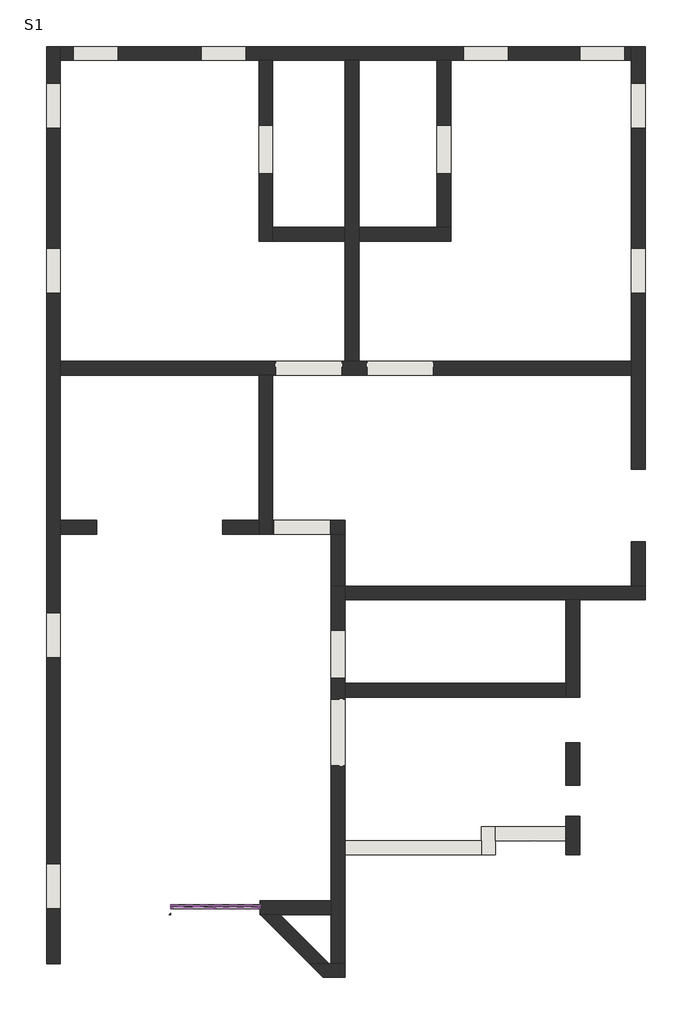
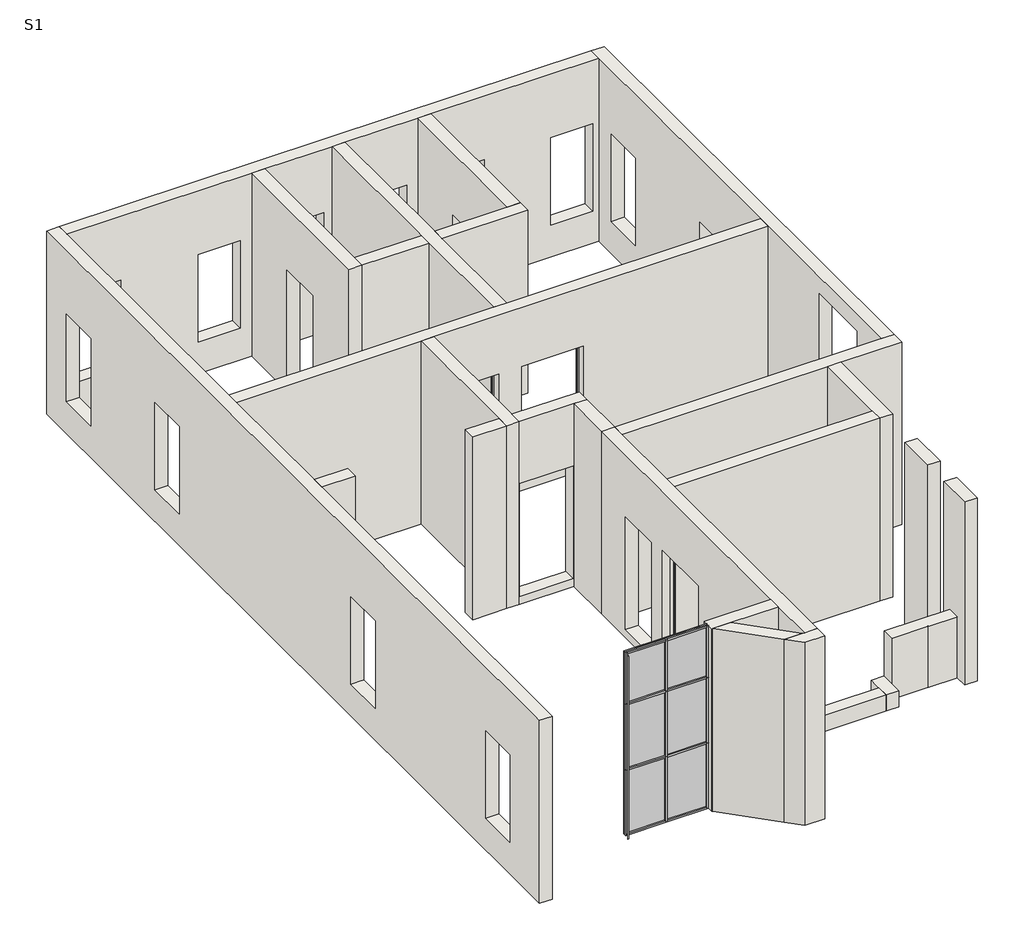
# One storey: 26 walls, 17 members, 6 plates.
"""IFC4 building model written with IfcOpenShell, lengths in millimetres."""

from ifc_helpers import new_model, si_unit, frame, origin, place, context, project, spatial, polyline, circle_curve, outline, extrude, faceted_brep, transform, mapped, element, save
from ifc_brep_helpers import plane_surface, revolved_surface, advanced_brep
from components import rectangular_mullion_30mm_square_a2edb205, rectangular_mullion_30mm_square_7d0e1db8, rectangular_mullion_30mm_square_4c7eb74d, rectangular_mullion_30mm_square_e6372653, rectangular_mullion_30mm_square_88df2287, rectangular_mullion_30mm_square_3df302c3, rectangular_mullion_30mm_square_038c5b05, rectangular_mullion_30mm_square_2b64bb93, system_panel_glazed_12388ada, system_panel_glazed_b614e8ed, system_panel_glazed_74337a84, system_panel_glazed_fe2b7919

model = new_model("IFC4")

# Units and contexts
model_context = context("Model", 3, world=origin())
ifc_project = project(units=[si_unit("LENGTHUNIT", "METRE", prefix="MILLI")], contexts=[model_context])

# Site, building, storey
site = spatial("IfcSite", under=ifc_project)
building = spatial("IfcBuilding", under=site)
storey = spatial("IfcBuildingStorey", under=building, Name="S1", Elevation=3750.0)

# Members
placement = place(None, origin())
rectangular_mullion_30mm_square_shape = rectangular_mullion_30mm_square_a2edb205(model_context)
element("IfcMember", 1, ObjectType="Rectangular Mullion : 30mm Square", at=placement, inside=storey, context=model_context, shape_type="MappedRepresentation", body=[
    mapped(rectangular_mullion_30mm_square_shape, transform((-6793.8712297, -9162.0014262, 7200.0), x_axis=(0.0, 0.0, 1.0), y_axis=(0.0, -1.0, 0.0), z_axis=(1.0, 0.0, 0.0))),
])
element("IfcMember", 2, ObjectType="Rectangular Mullion : 30mm Square", at=placement, inside=storey, context=model_context, shape_type="MappedRepresentation", body=[
    mapped(rectangular_mullion_30mm_square_shape, transform((-7498.8712297, -9162.0014262, 3750.0), x_axis=(0.0, 0.0, -1.0), y_axis=(0.0, -1.0, 0.0), z_axis=(-1.0, 0.0, 0.0))),
])
rectangular_mullion_30mm_square_2_shape = rectangular_mullion_30mm_square_7d0e1db8(model_context)
element("IfcMember", 3, ObjectType="Rectangular Mullion : 30mm Square", at=placement, inside=storey, context=model_context, shape_type="MappedRepresentation", body=[
    mapped(rectangular_mullion_30mm_square_2_shape, transform((-7513.8712297, -9162.0014262, 3750.0), x_axis=(1.0, 0.0, 0.0), y_axis=(0.0, -1.0, 0.0), z_axis=(0.0, 0.0, -1.0))),
])
rectangular_mullion_30mm_square_3_shape = rectangular_mullion_30mm_square_4c7eb74d(model_context)
element("IfcMember", 4, ObjectType="Rectangular Mullion : 30mm Square", at=placement, inside=storey, context=model_context, shape_type="MappedRepresentation", body=[
    mapped(rectangular_mullion_30mm_square_3_shape, transform((-6793.8712297, -9162.0014262, 6225.0), x_axis=(0.0, 0.0, 1.0), y_axis=(0.0, -1.0, 0.0), z_axis=(1.0, 0.0, 0.0))),
])
element("IfcMember", 5, ObjectType="Rectangular Mullion : 30mm Square", at=placement, inside=storey, context=model_context, shape_type="MappedRepresentation", body=[
    mapped(rectangular_mullion_30mm_square_3_shape, transform((-6793.8712297, -9162.0014262, 4987.5), x_axis=(0.0, 0.0, 1.0), y_axis=(0.0, -1.0, 0.0), z_axis=(1.0, 0.0, 0.0))),
])
element("IfcMember", 6, ObjectType="Rectangular Mullion : 30mm Square", at=placement, inside=storey, context=model_context, shape_type="MappedRepresentation", body=[
    mapped(rectangular_mullion_30mm_square_2_shape, transform((-7513.8712297, -9162.0014262, 4987.5), x_axis=(1.0, 0.0, 0.0), y_axis=(0.0, -1.0, 0.0), z_axis=(0.0, 0.0, -1.0))),
])
rectangular_mullion_30mm_square_4_shape = rectangular_mullion_30mm_square_e6372653(model_context)
element("IfcMember", 7, ObjectType="Rectangular Mullion : 30mm Square", at=placement, inside=storey, context=model_context, shape_type="MappedRepresentation", body=[
    mapped(rectangular_mullion_30mm_square_4_shape, transform((-6763.8712297, -9162.0014262, 3750.0), x_axis=(1.0, 0.0, 0.0), y_axis=(0.0, -1.0, 0.0), z_axis=(0.0, 0.0, -1.0))),
])
element("IfcMember", 8, ObjectType="Rectangular Mullion : 30mm Square", at=placement, inside=storey, context=model_context, shape_type="MappedRepresentation", body=[
    mapped(rectangular_mullion_30mm_square_4_shape, transform((-6763.8712297, -9162.0014262, 4987.5), x_axis=(1.0, 0.0, 0.0), y_axis=(0.0, -1.0, 0.0), z_axis=(0.0, 0.0, -1.0))),
])
element("IfcMember", 9, ObjectType="Rectangular Mullion : 30mm Square", at=placement, inside=storey, context=model_context, shape_type="MappedRepresentation", body=[
    mapped(rectangular_mullion_30mm_square_4_shape, transform((-8243.8712297, -9162.0014262, 6225.0), x_axis=(-1.0, 0.0, 0.0), y_axis=(0.0, -1.0, 0.0), z_axis=(0.0, 0.0, 1.0))),
])
element("IfcMember", 10, ObjectType="Rectangular Mullion : 30mm Square", at=placement, inside=storey, context=model_context, shape_type="MappedRepresentation", body=[
    mapped(rectangular_mullion_30mm_square_4_shape, transform((-8243.8712297, -9162.0014262, 4987.5), x_axis=(-1.0, 0.0, 0.0), y_axis=(0.0, -1.0, 0.0), z_axis=(0.0, 0.0, 1.0))),
])
rectangular_mullion_30mm_square_5_shape = rectangular_mullion_30mm_square_88df2287(model_context)
element("IfcMember", 11, ObjectType="Rectangular Mullion : 30mm Square", at=placement, inside=storey, context=model_context, shape_type="MappedRepresentation", body=[
    mapped(rectangular_mullion_30mm_square_5_shape, transform((-8213.8712297, -9162.0014262, 3750.0), x_axis=(0.0, 0.0, -1.0), y_axis=(0.0, -1.0, 0.0), z_axis=(-1.0, 0.0, 0.0))),
])
rectangular_mullion_30mm_square_6_shape = rectangular_mullion_30mm_square_3df302c3(model_context)
element("IfcMember", 12, ObjectType="Rectangular Mullion : 30mm Square", at=placement, inside=storey, context=model_context, shape_type="MappedRepresentation", body=[
    mapped(rectangular_mullion_30mm_square_6_shape, transform((-7528.8712297, -9162.0014262, 6225.0), x_axis=(0.0, 0.0, 1.0), y_axis=(0.0, -1.0, 0.0), z_axis=(1.0, 0.0, 0.0))),
])
element("IfcMember", 13, ObjectType="Rectangular Mullion : 30mm Square", at=placement, inside=storey, context=model_context, shape_type="MappedRepresentation", body=[
    mapped(rectangular_mullion_30mm_square_6_shape, transform((-7528.8712297, -9162.0014262, 4987.5), x_axis=(0.0, 0.0, 1.0), y_axis=(0.0, -1.0, 0.0), z_axis=(1.0, 0.0, 0.0))),
])
element("IfcMember", 14, ObjectType="Rectangular Mullion : 30mm Square", at=placement, inside=storey, context=model_context, shape_type="MappedRepresentation", body=[
    mapped(rectangular_mullion_30mm_square_5_shape, transform((-7528.8712297, -9162.0014262, 7200.0), x_axis=(0.0, 0.0, 1.0), y_axis=(0.0, -1.0, 0.0), z_axis=(1.0, 0.0, 0.0))),
])
rectangular_mullion_30mm_square_7_shape = rectangular_mullion_30mm_square_038c5b05(model_context)
element("IfcMember", 15, ObjectType="Rectangular Mullion : 30mm Square", at=placement, inside=storey, context=model_context, shape_type="MappedRepresentation", body=[
    mapped(rectangular_mullion_30mm_square_7_shape, transform((-7513.8712297, -9162.0014262, 6225.0), x_axis=(1.0, 0.0, 0.0), y_axis=(0.0, -1.0, 0.0), z_axis=(0.0, 0.0, -1.0))),
])
rectangular_mullion_30mm_square_8_shape = rectangular_mullion_30mm_square_2b64bb93(model_context)
element("IfcMember", 16, ObjectType="Rectangular Mullion : 30mm Square", at=placement, inside=storey, context=model_context, shape_type="MappedRepresentation", body=[
    mapped(rectangular_mullion_30mm_square_8_shape, transform((-8243.8712297, -9162.0014262, 7200.0), x_axis=(-1.0, 0.0, 0.0), y_axis=(0.0, -1.0, 0.0), z_axis=(0.0, 0.0, 1.0))),
])
element("IfcMember", 17, ObjectType="Rectangular Mullion : 30mm Square", at=placement, inside=storey, context=model_context, shape_type="MappedRepresentation", body=[
    mapped(rectangular_mullion_30mm_square_8_shape, transform((-6763.8712297, -9162.0014262, 6225.0), x_axis=(1.0, 0.0, 0.0), y_axis=(0.0, -1.0, 0.0), z_axis=(0.0, 0.0, -1.0))),
])

# Plates
system_panel_glazed_shape = system_panel_glazed_12388ada(model_context)
element("IfcPlate", 18, ObjectType="System Panel : Glazed", at=placement, inside=storey, context=model_context, shape_type="MappedRepresentation", body=[
    mapped(system_panel_glazed_shape, transform((-7138.8712297, -9162.0014262, 3750.0), x_axis=(1.0, 0.0, 0.0), y_axis=(0.0, 1.0, 0.0), z_axis=(0.0, 0.0, 1.0))),
])
element("IfcPlate", 19, ObjectType="System Panel : Glazed", at=placement, inside=storey, context=model_context, shape_type="MappedRepresentation", body=[
    mapped(system_panel_glazed_shape, transform((-7138.8712297, -9162.0014262, 4987.5), x_axis=(1.0, 0.0, 0.0), y_axis=(0.0, 1.0, 0.0), z_axis=(0.0, 0.0, 1.0))),
])
system_panel_glazed_2_shape = system_panel_glazed_b614e8ed(model_context)
element("IfcPlate", 20, ObjectType="System Panel : Glazed", at=placement, inside=storey, context=model_context, shape_type="MappedRepresentation", body=[
    mapped(system_panel_glazed_2_shape, transform((-7878.8712297, -9162.0014262, 3750.0), x_axis=(1.0, 0.0, 0.0), y_axis=(0.0, 1.0, 0.0), z_axis=(0.0, 0.0, 1.0))),
])
element("IfcPlate", 21, ObjectType="System Panel : Glazed", at=placement, inside=storey, context=model_context, shape_type="MappedRepresentation", body=[
    mapped(system_panel_glazed_2_shape, transform((-7878.8712297, -9162.0014262, 4987.5), x_axis=(1.0, 0.0, 0.0), y_axis=(0.0, 1.0, 0.0), z_axis=(0.0, 0.0, 1.0))),
])
system_panel_glazed_3_shape = system_panel_glazed_74337a84(model_context)
element("IfcPlate", 22, ObjectType="System Panel : Glazed", at=placement, inside=storey, context=model_context, shape_type="MappedRepresentation", body=[
    mapped(system_panel_glazed_3_shape, transform((-7878.8712297, -9162.0014262, 6225.0), x_axis=(1.0, 0.0, 0.0), y_axis=(0.0, 1.0, 0.0), z_axis=(0.0, 0.0, 1.0))),
])
system_panel_glazed_4_shape = system_panel_glazed_fe2b7919(model_context)
element("IfcPlate", 23, ObjectType="System Panel : Glazed", at=placement, inside=storey, context=model_context, shape_type="MappedRepresentation", body=[
    mapped(system_panel_glazed_4_shape, transform((-7138.8712297, -9162.0014262, 6225.0), x_axis=(1.0, 0.0, 0.0), y_axis=(0.0, 1.0, 0.0), z_axis=(0.0, 0.0, 1.0))),
])

# Walls
element("IfcWall", 24, ObjectType="230", at=placement, inside=storey, context=model_context, shape_type="Brep", body=[
    faceted_brep([(-10078.8712297, -10087.0014262, 3750.0), (-10078.8712297, -3817.0014262, 3750.0), (-10078.8712297, -2955.4326238, 3750.0), (-10078.8712297, -2725.4326238, 3750.0), (-10078.8712297, -317.0014262, 3750.0), (-10078.8712297, -87.0014262, 3750.0), (-10078.8712297, 4912.9985738, 3750.0), (-10078.8712297, 5142.9985738, 3750.0), (-10078.8712297, 5142.9985738, 7200.0), (-10078.8712297, 4912.9985738, 7200.0), (-10078.8712297, -87.0014262, 7200.0), (-10078.8712297, -317.0014262, 7200.0), (-10078.8712297, -2725.4326238, 7200.0), (-10078.8712297, -2955.4326238, 7200.0), (-10078.8712297, -10087.0014262, 7200.0), (-10078.8712297, 3782.9985738, 4350.0), (-10078.8712297, 3782.9985738, 6000.0), (-10078.8712297, 4532.9985738, 6000.0), (-10078.8712297, 4532.9985738, 4350.0), (-10078.8712297, 1042.9985738, 4350.0), (-10078.8712297, 1042.9985738, 6000.0), (-10078.8712297, 1792.9985738, 6000.0), (-10078.8712297, 1792.9985738, 4350.0), (-10078.8712297, -5007.0014262, 4350.0), (-10078.8712297, -5007.0014262, 6000.0), (-10078.8712297, -4257.0014262, 6000.0), (-10078.8712297, -4257.0014262, 4350.0), (-10078.8712297, -9177.0014262, 4350.0), (-10078.8712297, -9177.0014262, 6000.0), (-10078.8712297, -8427.0014262, 6000.0), (-10078.8712297, -8427.0014262, 4350.0), (-10308.8712297, -10087.0014262, 3750.0), (-10308.8712297, -10087.0014262, 7200.0), (-10308.8712297, 5142.9985738, 7200.0), (-10308.8712297, 5142.9985738, 3750.0), (-10308.8712297, -3817.0014262, 3750.0), (-10308.8712297, 3782.9985738, 4350.0), (-10308.8712297, 4532.9985738, 4350.0), (-10308.8712297, 4532.9985738, 6000.0), (-10308.8712297, 3782.9985738, 6000.0), (-10308.8712297, 1042.9985738, 4350.0), (-10308.8712297, 1792.9985738, 4350.0), (-10308.8712297, 1792.9985738, 6000.0), (-10308.8712297, 1042.9985738, 6000.0), (-10308.8712297, -5007.0014262, 4350.0), (-10308.8712297, -4257.0014262, 4350.0), (-10308.8712297, -4257.0014262, 6000.0), (-10308.8712297, -5007.0014262, 6000.0), (-10308.8712297, -9177.0014262, 4350.0), (-10308.8712297, -8427.0014262, 4350.0), (-10308.8712297, -8427.0014262, 6000.0), (-10308.8712297, -9177.0014262, 6000.0)], [[[0, 1, 2, 3, 4, 5, 6, 7, 8, 9, 10, 11, 12, 13, 14], [15, 16, 17, 18], [19, 20, 21, 22], [23, 24, 25, 26], [27, 28, 29, 30]], [[31, 32, 33, 34, 35], [36, 37, 38, 39], [40, 41, 42, 43], [44, 45, 46, 47], [48, 49, 50, 51]], [[7, 6, 5, 4, 3, 2, 1, 0, 31, 35, 34]], [[14, 13, 12, 11, 10, 9, 8, 33, 32]], [[8, 7, 34, 33]], [[0, 14, 32, 31]], [[16, 15, 36, 39]], [[17, 16, 39, 38]], [[18, 17, 38, 37]], [[15, 18, 37, 36]], [[20, 19, 40, 43]], [[21, 20, 43, 42]], [[22, 21, 42, 41]], [[19, 22, 41, 40]], [[24, 23, 44, 47]], [[25, 24, 47, 46]], [[26, 25, 46, 45]], [[23, 26, 45, 44]], [[28, 27, 48, 51]], [[29, 28, 51, 50]], [[30, 29, 50, 49]], [[27, 30, 49, 48]]]),
])
element("IfcWall", 25, ObjectType="230", at=placement, inside=storey, context=model_context, shape_type="SweptSolid", body=[
    extrude(outline(polyline([(-9478.8712297, -2955.4326238), (-10078.8712297, -2955.4326238), (-10078.8712297, -2725.4326238), (-9478.8712297, -2725.4326238), (-9478.8712297, -2955.4326238)])), frame((0.0, 0.0, 3750.0), z_axis=(0.0, 0.0, 1.0), x_axis=(1.0, 0.0, 0.0)), (0.0, 0.0, 1.0), 3450.0),
])
element("IfcWall", 26, ObjectType="230", at=placement, inside=storey, context=model_context, shape_type="Brep", body=[
    faceted_brep([(-5578.8712297, -3817.0014262, 3750.0), (-5578.8712297, -9047.0014262, 3750.0), (-5578.8712297, -9277.0014262, 3750.0), (-5578.8712297, -10087.0014262, 3750.0), (-5578.8712297, -10087.0014262, 7200.0), (-5578.8712297, -9277.0014262, 7200.0), (-5578.8712297, -9047.0014262, 7200.0), (-5578.8712297, -3817.0014262, 7200.0), (-5578.8712297, -5347.0014262, 6025.0), (-5578.8712297, -5347.0014262, 3900.0), (-5578.8712297, -4547.0014262, 3900.0), (-5578.8712297, -4547.0014262, 6025.0), (-5578.8712297, -5694.7514262, 6089.5), (-5578.8712297, -6799.2514262, 6089.5), (-5578.8712297, -6799.2514262, 3900.0), (-5578.8712297, -5694.7514262, 3900.0), (-5348.8712297, -10087.0014262, 3750.0), (-5348.8712297, -8277.0014262, 3750.0), (-5348.8712297, -8047.0014262, 3750.0), (-5348.8712297, -5662.0014262, 3750.0), (-5348.8712297, -5432.0014262, 3750.0), (-5348.8712297, -4047.0014262, 3750.0), (-5348.8712297, -3817.0014262, 3750.0), (-5348.8712297, -3817.0014262, 7200.0), (-5348.8712297, -4047.0014262, 7200.0), (-5348.8712297, -5432.0014262, 7200.0), (-5348.8712297, -5662.0014262, 7200.0), (-5348.8712297, -10087.0014262, 7200.0), (-5348.8712297, -5347.0014262, 3900.0), (-5348.8712297, -5347.0014262, 6025.0), (-5348.8712297, -4547.0014262, 6025.0), (-5348.8712297, -4547.0014262, 3900.0), (-5348.8712297, -6799.2514262, 6089.5), (-5348.8712297, -5694.7514262, 6089.5), (-5348.8712297, -5694.7514262, 3900.0), (-5348.8712297, -6799.2514262, 3900.0), (-5368.8712297, -6799.2514262, 6089.5), (-5368.8712297, -5694.7514262, 6089.5), (-5445.8712297, -5694.7514262, 6089.5), (-5445.8712297, -6799.2514262, 6089.5), (-5368.8712297, -5694.7514262, 3900.0), (-5445.8712297, -5694.7514262, 3900.0), (-5368.8712297, -5679.7514262, 3900.0), (-5445.8712297, -5679.7514262, 3900.0), (-5445.8712297, -6799.2514262, 3900.0), (-5445.8712297, -6814.2514262, 3900.0), (-5368.8712297, -6814.2514262, 3900.0), (-5368.8712297, -6799.2514262, 3900.0), (-5368.8712297, -6814.2514262, 6104.5), (-5445.8712297, -6814.2514262, 6104.5), (-5445.8712297, -5679.7514262, 6104.5), (-5368.8712297, -5679.7514262, 6104.5)], [[[0, 1, 2, 3, 4, 5, 6, 7], [8, 9, 10, 11], [12, 13, 14, 15]], [[16, 17, 18, 19, 20, 21, 22, 23, 24, 25, 26, 27], [28, 29, 30, 31], [32, 33, 34, 35]], [[3, 2, 1, 0, 22, 21, 20, 19, 18, 17, 16]], [[7, 6, 5, 4, 27, 26, 25, 24, 23]], [[4, 3, 16, 27]], [[29, 28, 9, 8]], [[30, 29, 8, 11]], [[31, 30, 11, 10]], [[28, 31, 10, 9]], [[0, 7, 23, 22]], [[32, 36, 37, 33]], [[12, 38, 39, 13]], [[33, 37, 40, 34]], [[38, 12, 15, 41]], [[34, 40, 42, 43, 41, 15, 14, 44, 45, 46, 47, 35]], [[36, 32, 35, 47]], [[13, 39, 44, 14]], [[48, 49, 50, 51]], [[43, 42, 51, 50]], [[39, 38, 41, 43, 50, 49, 45, 44]], [[46, 45, 49, 48]], [[37, 36, 47, 46, 48, 51, 42, 40]]]),
])
element("IfcWall", 27, ObjectType="230", at=placement, inside=storey, context=model_context, shape_type="Brep", body=[
    faceted_brep([(-5348.8712297, -10087.0014262, 3750.0), (-5578.8712297, -10087.0014262, 3750.0), (-5616.23667, -10087.0014262, 3750.0), (-5941.5057893, -10087.0014262, 3750.0), (-5941.5057893, -10087.0014262, 7200.0), (-5616.23667, -10087.0014262, 7200.0), (-5578.8712297, -10087.0014262, 7200.0), (-5348.8712297, -10087.0014262, 7200.0), (-5348.8712297, -10317.0014262, 3750.0), (-5348.8712297, -10317.0014262, 7200.0), (-5711.5057893, -10317.0014262, 7200.0), (-5711.5057893, -10317.0014262, 3750.0)], [[[0, 1, 2, 3, 4, 5, 6, 7]], [[8, 9, 10, 11]], [[3, 2, 1, 0, 8, 11]], [[7, 6, 5, 4, 10, 9]], [[0, 7, 9, 8]], [[4, 3, 11, 10]]]),
])
element("IfcWall", 28, ObjectType="230", at=placement, inside=storey, context=model_context, shape_type="SweptSolid", body=[
    extrude(outline(polyline([(-6426.23667, -9277.0014262), (-5616.23667, -10087.0014262), (-5941.5057893, -10087.0014262), (-6751.5057893, -9277.0014262), (-6426.23667, -9277.0014262)])), frame((0.0, 0.0, 3750.0), z_axis=(0.0, 0.0, 1.0), x_axis=(1.0, 0.0, 0.0)), (0.0, 0.0, 1.0), 3450.0),
])
element("IfcWall", 29, ObjectType="230", at=placement, inside=storey, context=model_context, shape_type="Brep", body=[
    faceted_brep([(-5578.8712297, -9047.0014262, 7200.0), (-5578.8712297, -9047.0014262, 3750.0), (-6763.8712297, -9047.0014262, 3750.0), (-6763.8712297, -9047.0014262, 7200.0), (-5578.8712297, -9277.0014262, 3750.0), (-5578.8712297, -9277.0014262, 7200.0), (-6426.23667, -9277.0014262, 7200.0), (-6751.5057893, -9277.0014262, 7200.0), (-6763.8712297, -9277.0014262, 7200.0), (-6763.8712297, -9277.0014262, 3750.0), (-6751.5057893, -9277.0014262, 3750.0), (-6426.23667, -9277.0014262, 3750.0)], [[[0, 1, 2, 3]], [[4, 5, 6, 7, 8, 9, 10, 11]], [[1, 4, 11, 10, 9, 2]], [[5, 0, 3, 8, 7, 6]], [[3, 2, 9, 8]], [[1, 0, 5, 4]]]),
    faceted_brep([(-8268.1448516, -9277.0014262, 7200.0), (-8268.1448516, -9277.0014262, 3750.0), (-8243.8712297, -9277.0014262, 3750.0), (-8243.8712297, -9277.0014262, 7200.0), (-8243.8712297, -9252.7278043, 3750.0), (-8243.8712297, -9252.7278043, 7200.0)], [[[0, 1, 2, 3]], [[2, 1, 4]], [[0, 3, 5]], [[3, 2, 4, 5]], [[1, 0, 5, 4]]]),
])
element("IfcWall", 30, ObjectType="230", at=placement, inside=storey, context=model_context, shape_type="AdvancedBrep", body=[
    advanced_brep(
    [(-1678.8712297, -8047.0014262, 3750.0), (-1678.8712297, -8047.0014262, 4900.0), (-2191.3712297, -8047.0014262, 4900.0), (-2191.3712297, -8047.0014262, 3750.0), (-2848.8712297, -8047.0014262, 4900.0), (-2848.8712297, -8047.0014262, 3750.0), (-2206.3712297, -8047.0014262, 3750.0), (-2206.3712297, -8047.0014262, 4900.0), (-1678.8712297, -7817.0014262, 3750.0), (-2848.8712297, -7817.0014262, 3750.0), (-2848.8712297, -7817.0014262, 4050.0), (-2848.8712297, -7817.0014262, 4900.0), (-1678.8712297, -7817.0014262, 4900.0), (-2198.8712297, -8039.5014262, 3750.0), (-2198.8712297, -8039.5014262, 4900.0)],
    [
        (0, 1),
        (1, 2),
        (2, 3),
        (3, 0),
        (4, 5),
        (5, 6),
        (6, 7),
        (7, 4),
        (8, 9),
        (9, 10),
        (10, 11),
        (11, 12),
        (12, 8),
        (8, 0),
        (3, 13, circle_curve(frame((-2198.8712297, -8047.0014262, 3750.0), z_axis=(0.0, 0.0, 1.0), x_axis=(0.0, 1.0, 0.0)), 7.5)),
        (13, 6, circle_curve(frame((-2198.8712297, -8047.0014262, 3750.0), z_axis=(0.0, 0.0, 1.0), x_axis=(0.0, 1.0, 0.0)), 7.5)),
        (5, 9),
        (11, 4),
        (7, 14, circle_curve(frame((-2198.8712297, -8047.0014262, 4900.0), z_axis=(0.0, 0.0, -1.0), x_axis=(0.0, 1.0, 0.0)), 7.5)),
        (14, 2, circle_curve(frame((-2198.8712297, -8047.0014262, 4900.0), z_axis=(0.0, 0.0, -1.0), x_axis=(0.0, 1.0, 0.0)), 7.5)),
        (1, 12),
        (14, 13),
    ],
    [
        plane_surface(frame((-2963.8712297, -8047.0014262, 3750.0), z_axis=(0.0, -1.0, 0.0), x_axis=(1.0, 0.0, 0.0))),
        plane_surface(frame((-2963.8712297, -7817.0014262, 3750.0), z_axis=(0.0, 1.0, 0.0), x_axis=(-1.0, 0.0, 0.0))),
        plane_surface(frame((-2963.8712297, -8047.0014262, 3750.0), z_axis=(0.0, 0.0, -1.0), x_axis=(0.0, 1.0, 0.0))),
        plane_surface(frame((-1563.8712297, -8047.0014262, 4900.0), z_axis=(0.0, 0.0, 1.0), x_axis=(0.0, 1.0, 0.0))),
        plane_surface(frame((-1678.8712297, -8592.0014262, 3750.0), z_axis=(1.0, 0.0, 0.0), x_axis=(0.0, -1.0, 0.0))),
        plane_surface(frame((-2848.8712297, -8047.0014262, 3750.0), z_axis=(-1.0, 0.0, 0.0), x_axis=(0.0, 1.0, 0.0))),
        revolved_surface(polyline([(-2198.8712297, -8039.5014262, 4900.0), (-2198.8712297, -8039.5014262, 3750.0)]), (-2198.8712297, -8047.0014262, 4900.0), (0.0, 0.0, 1.0)),
    ],
    [
        (0, [[1, 2, 3, 4]]),
        (0, [[5, 6, 7, 8]]),
        (1, [[9, 10, 11, 12, 13]]),
        (2, [[-9, 14, -4, 15, 16, -6, 17]]),
        (3, [[-12, 18, -8, 19, 20, -2, 21]]),
        (4, [[-1, -14, -13, -21]]),
        (5, [[-5, -18, -11, -10, -17]]),
        (6, [[22, -15, -3, -20]]),
        (6, [[-22, -19, -7, -16]]),
    ],
),
])
element("IfcWall", 31, ObjectType="230", at=placement, inside=storey, context=model_context, shape_type="SweptSolid", body=[
    extrude(outline(polyline([(-3078.8712297, -8277.0014262), (-5348.8712297, -8277.0014262), (-5348.8712297, -8047.0014262), (-3078.8712297, -8047.0014262), (-3078.8712297, -8277.0014262)])), frame((0.0, 0.0, 3750.0), z_axis=(0.0, 0.0, 1.0), x_axis=(1.0, 0.0, 0.0)), (0.0, 0.0, 1.0), 300.0),
])
element("IfcWall", 32, ObjectType="230", at=placement, inside=storey, context=model_context, shape_type="Brep", body=[
    faceted_brep([(-1678.8712297, -7637.0014262, 3750.0), (-1678.8712297, -7817.0014262, 3750.0), (-1678.8712297, -8047.0014262, 3750.0), (-1678.8712297, -8277.0014262, 3750.0), (-1678.8712297, -8277.0014262, 7200.0), (-1678.8712297, -7637.0014262, 7200.0), (-1448.8712297, -7637.0014262, 3750.0), (-1448.8712297, -7637.0014262, 7200.0), (-1448.8712297, -8277.0014262, 7200.0), (-1448.8712297, -8277.0014262, 3750.0)], [[[0, 1, 2, 3, 4, 5]], [[6, 7, 8, 9]], [[3, 2, 1, 0, 6, 9]], [[4, 3, 9, 8]], [[5, 4, 8, 7]], [[0, 5, 7, 6]]]),
])
element("IfcWall", 33, ObjectType="230", at=placement, inside=storey, context=model_context, shape_type="SweptSolid", body=[
    extrude(outline(polyline([(-1448.8712297, -6422.0014262), (-1448.8712297, -7122.0014262), (-1678.8712297, -7122.0014262), (-1678.8712297, -6422.0014262), (-1448.8712297, -6422.0014262)])), frame((0.0, 0.0, 3750.0), z_axis=(0.0, 0.0, 1.0), x_axis=(1.0, 0.0, 0.0)), (0.0, 0.0, 1.0), 3450.0),
])
element("IfcWall", 34, ObjectType="230", at=placement, inside=storey, context=model_context, shape_type="Brep", body=[
    faceted_brep([(-1448.8712297, -5662.0014262, 3750.0), (-1448.8712297, -4047.0014262, 3750.0), (-1448.8712297, -4047.0014262, 7200.0), (-1448.8712297, -5662.0014262, 7200.0), (-1448.8712297, -4289.5014262, 5400.0), (-1448.8712297, -5189.5014262, 5400.0), (-1448.8712297, -5189.5014262, 6000.0), (-1448.8712297, -4289.5014262, 6000.0), (-1678.8712297, -5662.0014262, 3750.0), (-1678.8712297, -5662.0014262, 7200.0), (-1678.8712297, -5432.0014262, 7200.0), (-1678.8712297, -4047.0014262, 7200.0), (-1678.8712297, -4047.0014262, 3750.0), (-1678.8712297, -5432.0014262, 3750.0), (-1678.8712297, -4289.5014262, 5400.0), (-1678.8712297, -4289.5014262, 6000.0), (-1678.8712297, -5189.5014262, 6000.0), (-1678.8712297, -5189.5014262, 5400.0)], [[[0, 1, 2, 3], [4, 5, 6, 7]], [[8, 9, 10, 11, 12, 13], [14, 15, 16, 17]], [[1, 0, 8, 13, 12]], [[3, 2, 11, 10, 9]], [[2, 1, 12, 11]], [[0, 3, 9, 8]], [[15, 14, 4, 7]], [[16, 15, 7, 6]], [[17, 16, 6, 5]], [[14, 17, 5, 4]]]),
])
element("IfcWall", 35, ObjectType="230", at=placement, inside=storey, context=model_context, shape_type="Brep", body=[
    faceted_brep([(-2848.8712297, -8277.0014262, 3750.0), (-2848.8712297, -8047.0014262, 3750.0), (-2848.8712297, -7817.0014262, 3750.0), (-2848.8712297, -7817.0014262, 4050.0), (-2848.8712297, -8277.0014262, 4050.0), (-3078.8712297, -8277.0014262, 3750.0), (-3078.8712297, -8277.0014262, 4050.0), (-3078.8712297, -8047.0014262, 4050.0), (-3078.8712297, -7817.0014262, 4050.0), (-3078.8712297, -7817.0014262, 3750.0), (-3078.8712297, -8047.0014262, 3750.0)], [[[0, 1, 2, 3, 4]], [[5, 6, 7, 8, 9, 10]], [[2, 1, 0, 5, 10, 9]], [[4, 3, 8, 7, 6]], [[0, 4, 6, 5]], [[3, 2, 9, 8]]]),
])
element("IfcWall", 36, ObjectType="230", at=placement, inside=storey, context=model_context, shape_type="SweptSolid", body=[
    extrude(outline(polyline([(-5348.8712297, -5432.0014262), (-1678.8712297, -5432.0014262), (-1678.8712297, -5662.0014262), (-5348.8712297, -5662.0014262), (-5348.8712297, -5432.0014262)])), frame((0.0, 0.0, 3750.0), z_axis=(0.0, 0.0, 1.0), x_axis=(1.0, 0.0, 0.0)), (0.0, 0.0, 1.0), 3450.0),
])
element("IfcWall", 37, ObjectType="230", at=placement, inside=storey, context=model_context, shape_type="Brep", body=[
    faceted_brep([(-6778.8712297, -317.0014262, 3750.0), (-6778.8712297, -2725.4326238, 3750.0), (-6778.8712297, -2955.4326238, 3750.0), (-6778.8712297, -2955.4326238, 7200.0), (-6778.8712297, -2725.4326238, 7200.0), (-6778.8712297, -317.0014262, 7200.0), (-6548.8712297, -317.0014262, 3750.0), (-6548.8712297, -317.0014262, 7200.0), (-6548.8712297, -2725.4326238, 7200.0), (-6548.8712297, -2955.4326238, 7200.0), (-6548.8712297, -2955.4326238, 3750.0), (-6548.8712297, -2725.4326238, 3750.0)], [[[0, 1, 2, 3, 4, 5]], [[6, 7, 8, 9, 10, 11]], [[2, 1, 0, 6, 11, 10]], [[5, 4, 3, 9, 8, 7]], [[0, 5, 7, 6]], [[3, 2, 10, 9]]]),
])
element("IfcWall", 38, ObjectType="230", at=placement, inside=storey, context=model_context, shape_type="Brep", body=[
    faceted_brep([(-588.8712297, -87.0014262, 3750.0), (-5118.8712297, -87.0014262, 3750.0), (-5348.8712297, -87.0014262, 3750.0), (-10078.8712297, -87.0014262, 3750.0), (-10078.8712297, -87.0014262, 7200.0), (-5348.8712297, -87.0014262, 7200.0), (-5118.8712297, -87.0014262, 7200.0), (-588.8712297, -87.0014262, 7200.0), (-5396.6212297, -87.0014262, 6089.5), (-6501.1212297, -87.0014262, 6089.5), (-6501.1212297, -87.0014262, 3900.0), (-5396.6212297, -87.0014262, 3900.0), (-3881.6212297, -87.0014262, 6089.5), (-4986.1212297, -87.0014262, 6089.5), (-4986.1212297, -87.0014262, 3900.0), (-3881.6212297, -87.0014262, 3900.0), (-10078.8712297, -317.0014262, 3750.0), (-6778.8712297, -317.0014262, 3750.0), (-6548.8712297, -317.0014262, 3750.0), (-588.8712297, -317.0014262, 3750.0), (-588.8712297, -317.0014262, 7200.0), (-6548.8712297, -317.0014262, 7200.0), (-6778.8712297, -317.0014262, 7200.0), (-10078.8712297, -317.0014262, 7200.0), (-6501.1212297, -317.0014262, 6089.5), (-5396.6212297, -317.0014262, 6089.5), (-5396.6212297, -317.0014262, 3900.0), (-6501.1212297, -317.0014262, 3900.0), (-4986.1212297, -317.0014262, 6089.5), (-3881.6212297, -317.0014262, 6089.5), (-3881.6212297, -317.0014262, 3900.0), (-4986.1212297, -317.0014262, 3900.0), (-5396.6212297, -107.0014262, 6089.5), (-6501.1212297, -107.0014262, 6089.5), (-6501.1212297, -184.0014262, 6089.5), (-5396.6212297, -184.0014262, 6089.5), (-5396.6212297, -107.0014262, 3900.0), (-5396.6212297, -184.0014262, 3900.0), (-6501.1212297, -107.0014262, 3900.0), (-6516.1212297, -107.0014262, 3900.0), (-6516.1212297, -184.0014262, 3900.0), (-6501.1212297, -184.0014262, 3900.0), (-5381.6212297, -184.0014262, 3900.0), (-5381.6212297, -107.0014262, 3900.0), (-6516.1212297, -107.0014262, 6104.5), (-5381.6212297, -107.0014262, 6104.5), (-5381.6212297, -184.0014262, 6104.5), (-6516.1212297, -184.0014262, 6104.5), (-3881.6212297, -107.0014262, 6089.5), (-4986.1212297, -107.0014262, 6089.5), (-4986.1212297, -184.0014262, 6089.5), (-3881.6212297, -184.0014262, 6089.5), (-4986.1212297, -107.0014262, 3900.0), (-4986.1212297, -184.0014262, 3900.0), (-5001.1212297, -107.0014262, 3900.0), (-5001.1212297, -184.0014262, 3900.0), (-3881.6212297, -184.0014262, 3900.0), (-3866.6212297, -184.0014262, 3900.0), (-3866.6212297, -107.0014262, 3900.0), (-3881.6212297, -107.0014262, 3900.0), (-3866.6212297, -107.0014262, 6104.5), (-3866.6212297, -184.0014262, 6104.5), (-5001.1212297, -184.0014262, 6104.5), (-5001.1212297, -107.0014262, 6104.5)], [[[0, 1, 2, 3, 4, 5, 6, 7], [8, 9, 10, 11], [12, 13, 14, 15]], [[16, 17, 18, 19, 20, 21, 22, 23], [24, 25, 26, 27], [28, 29, 30, 31]], [[3, 2, 1, 0, 19, 18, 17, 16]], [[7, 6, 5, 4, 23, 22, 21, 20]], [[4, 3, 16, 23]], [[0, 7, 20, 19]], [[8, 32, 33, 9]], [[24, 34, 35, 25]], [[32, 8, 11, 36]], [[25, 35, 37, 26]], [[36, 11, 10, 38, 39, 40, 41, 27, 26, 37, 42, 43]], [[9, 33, 38, 10]], [[34, 24, 27, 41]], [[44, 45, 46, 47]], [[43, 42, 46, 45]], [[35, 34, 41, 40, 47, 46, 42, 37]], [[40, 39, 44, 47]], [[33, 32, 36, 43, 45, 44, 39, 38]], [[12, 48, 49, 13]], [[28, 50, 51, 29]], [[13, 49, 52, 14]], [[50, 28, 31, 53]], [[14, 52, 54, 55, 53, 31, 30, 56, 57, 58, 59, 15]], [[48, 12, 15, 59]], [[29, 51, 56, 30]], [[60, 61, 62, 63]], [[55, 54, 63, 62]], [[51, 50, 53, 55, 62, 61, 57, 56]], [[58, 57, 61, 60]], [[49, 48, 59, 58, 60, 63, 54, 52]]]),
])
element("IfcWall", 39, ObjectType="230", at=placement, inside=storey, context=model_context, shape_type="Brep", body=[
    faceted_brep([(-358.8712297, 5142.9985738, 7200.0), (-358.8712297, -3817.0014262, 7200.0), (-358.8712297, -3817.0014262, 3750.0), (-358.8712297, -3080.571442, 3750.0), (-358.8712297, -3080.571442, 6900.0), (-358.8712297, -1880.571442, 6900.0), (-358.8712297, -1880.571442, 3750.0), (-358.8712297, 5142.9985738, 3750.0), (-358.8712297, 4532.9985738, 4350.0), (-358.8712297, 3782.9985738, 4350.0), (-358.8712297, 3782.9985738, 6000.0), (-358.8712297, 4532.9985738, 6000.0), (-358.8712297, 1792.9985738, 4350.0), (-358.8712297, 1042.9985738, 4350.0), (-358.8712297, 1042.9985738, 6000.0), (-358.8712297, 1792.9985738, 6000.0), (-588.8712297, -3817.0014262, 7200.0), (-588.8712297, -317.0014262, 7200.0), (-588.8712297, -87.0014262, 7200.0), (-588.8712297, 4912.9985738, 7200.0), (-588.8712297, 5142.9985738, 7200.0), (-588.8712297, 5142.9985738, 3750.0), (-588.8712297, 4912.9985738, 3750.0), (-588.8712297, -87.0014262, 3750.0), (-588.8712297, -317.0014262, 3750.0), (-588.8712297, -1880.571442, 3750.0), (-588.8712297, -1880.571442, 6900.0), (-588.8712297, -3080.571442, 6900.0), (-588.8712297, -3080.571442, 3750.0), (-588.8712297, -3817.0014262, 3750.0), (-588.8712297, 4532.9985738, 4350.0), (-588.8712297, 4532.9985738, 6000.0), (-588.8712297, 3782.9985738, 6000.0), (-588.8712297, 3782.9985738, 4350.0), (-588.8712297, 1792.9985738, 4350.0), (-588.8712297, 1792.9985738, 6000.0), (-588.8712297, 1042.9985738, 6000.0), (-588.8712297, 1042.9985738, 4350.0)], [[[0, 1, 2, 3, 4, 5, 6, 7], [8, 9, 10, 11], [12, 13, 14, 15]], [[16, 17, 18, 19, 20, 21, 22, 23, 24, 25, 26, 27, 28, 29], [30, 31, 32, 33], [34, 35, 36, 37]], [[21, 7, 6, 25, 24, 23, 22]], [[2, 29, 28, 3]], [[1, 0, 20, 19, 18, 17, 16]], [[0, 7, 21, 20]], [[2, 1, 16, 29]], [[31, 30, 8, 11]], [[32, 31, 11, 10]], [[33, 32, 10, 9]], [[30, 33, 9, 8]], [[35, 34, 12, 15]], [[36, 35, 15, 14]], [[37, 36, 14, 13]], [[34, 37, 13, 12]], [[5, 26, 25, 6]], [[26, 5, 4, 27]], [[27, 4, 3, 28]]]),
])
element("IfcWall", 40, ObjectType="230", at=placement, inside=storey, context=model_context, shape_type="Brep", body=[
    faceted_brep([(-10078.8712297, 4912.9985738, 3750.0), (-6778.8712297, 4912.9985738, 3750.0), (-6548.8712297, 4912.9985738, 3750.0), (-5348.8712297, 4912.9985738, 3750.0), (-5118.8712297, 4912.9985738, 3750.0), (-3818.8712297, 4912.9985738, 3750.0), (-3588.8712297, 4912.9985738, 3750.0), (-588.8712297, 4912.9985738, 3750.0), (-588.8712297, 4912.9985738, 7200.0), (-3588.8712297, 4912.9985738, 7200.0), (-3818.8712297, 4912.9985738, 7200.0), (-5118.8712297, 4912.9985738, 7200.0), (-5348.8712297, 4912.9985738, 7200.0), (-6548.8712297, 4912.9985738, 7200.0), (-6778.8712297, 4912.9985738, 7200.0), (-10078.8712297, 4912.9985738, 7200.0), (-7738.8712297, 4912.9985738, 4350.0), (-7738.8712297, 4912.9985738, 6000.0), (-6988.8712297, 4912.9985738, 6000.0), (-6988.8712297, 4912.9985738, 4350.0), (-9868.8712297, 4912.9985738, 4350.0), (-9868.8712297, 4912.9985738, 6000.0), (-9118.8712297, 4912.9985738, 6000.0), (-9118.8712297, 4912.9985738, 4350.0), (-3378.8712297, 4912.9985738, 4350.0), (-3378.8712297, 4912.9985738, 6000.0), (-2628.8712297, 4912.9985738, 6000.0), (-2628.8712297, 4912.9985738, 4350.0), (-1448.8712297, 4912.9985738, 4350.0), (-1448.8712297, 4912.9985738, 6000.0), (-698.8712297, 4912.9985738, 6000.0), (-698.8712297, 4912.9985738, 4350.0), (-4918.8712297, 4912.9985738, 5400.0), (-4918.8712297, 4912.9985738, 6000.0), (-4018.8712297, 4912.9985738, 6000.0), (-4018.8712297, 4912.9985738, 5400.0), (-6398.8712297, 4912.9985738, 5400.0), (-6398.8712297, 4912.9985738, 6000.0), (-5498.8712297, 4912.9985738, 6000.0), (-5498.8712297, 4912.9985738, 5400.0), (-10078.8712297, 5142.9985738, 3750.0), (-10078.8712297, 5142.9985738, 7200.0), (-588.8712297, 5142.9985738, 7200.0), (-588.8712297, 5142.9985738, 3750.0), (-7738.8712297, 5142.9985738, 4350.0), (-6988.8712297, 5142.9985738, 4350.0), (-6988.8712297, 5142.9985738, 6000.0), (-7738.8712297, 5142.9985738, 6000.0), (-9868.8712297, 5142.9985738, 4350.0), (-9118.8712297, 5142.9985738, 4350.0), (-9118.8712297, 5142.9985738, 6000.0), (-9868.8712297, 5142.9985738, 6000.0), (-3378.8712297, 5142.9985738, 4350.0), (-2628.8712297, 5142.9985738, 4350.0), (-2628.8712297, 5142.9985738, 6000.0), (-3378.8712297, 5142.9985738, 6000.0), (-1448.8712297, 5142.9985738, 4350.0), (-698.8712297, 5142.9985738, 4350.0), (-698.8712297, 5142.9985738, 6000.0), (-1448.8712297, 5142.9985738, 6000.0), (-4918.8712297, 5142.9985738, 5400.0), (-4018.8712297, 5142.9985738, 5400.0), (-4018.8712297, 5142.9985738, 6000.0), (-4918.8712297, 5142.9985738, 6000.0), (-6398.8712297, 5142.9985738, 5400.0), (-5498.8712297, 5142.9985738, 5400.0), (-5498.8712297, 5142.9985738, 6000.0), (-6398.8712297, 5142.9985738, 6000.0)], [[[0, 1, 2, 3, 4, 5, 6, 7, 8, 9, 10, 11, 12, 13, 14, 15], [16, 17, 18, 19], [20, 21, 22, 23], [24, 25, 26, 27], [28, 29, 30, 31], [32, 33, 34, 35], [36, 37, 38, 39]], [[40, 41, 42, 43], [44, 45, 46, 47], [48, 49, 50, 51], [52, 53, 54, 55], [56, 57, 58, 59], [60, 61, 62, 63], [64, 65, 66, 67]], [[7, 6, 5, 4, 3, 2, 1, 0, 40, 43]], [[15, 14, 13, 12, 11, 10, 9, 8, 42, 41]], [[0, 15, 41, 40]], [[8, 7, 43, 42]], [[17, 16, 44, 47]], [[18, 17, 47, 46]], [[19, 18, 46, 45]], [[16, 19, 45, 44]], [[21, 20, 48, 51]], [[22, 21, 51, 50]], [[23, 22, 50, 49]], [[20, 23, 49, 48]], [[25, 24, 52, 55]], [[26, 25, 55, 54]], [[27, 26, 54, 53]], [[24, 27, 53, 52]], [[29, 28, 56, 59]], [[30, 29, 59, 58]], [[31, 30, 58, 57]], [[28, 31, 57, 56]], [[33, 32, 60, 63]], [[34, 33, 63, 62]], [[35, 34, 62, 61]], [[32, 35, 61, 60]], [[37, 36, 64, 67]], [[38, 37, 67, 66]], [[39, 38, 66, 65]], [[36, 39, 65, 64]]]),
])
element("IfcWall", 41, ObjectType="230", at=placement, inside=storey, context=model_context, shape_type="SweptSolid", body=[
    extrude(outline(polyline([(-6778.8712297, -2955.4326238), (-7378.8712297, -2955.4326238), (-7378.8712297, -2725.4326238), (-6778.8712297, -2725.4326238), (-6778.8712297, -2955.4326238)])), frame((0.0, 0.0, 3750.0), z_axis=(0.0, 0.0, 1.0), x_axis=(1.0, 0.0, 0.0)), (0.0, 0.0, 1.0), 3450.0),
])
element("IfcWall", 42, ObjectType="230", at=placement, inside=storey, context=model_context, shape_type="Brep", body=[
    faceted_brep([(-5118.8712297, -87.0014262, 3750.0), (-5118.8712297, 1912.9985738, 3750.0), (-5118.8712297, 2142.9985738, 3750.0), (-5118.8712297, 4912.9985738, 3750.0), (-5118.8712297, 4912.9985738, 7200.0), (-5118.8712297, 2142.9985738, 7200.0), (-5118.8712297, 1912.9985738, 7200.0), (-5118.8712297, -87.0014262, 7200.0), (-5348.8712297, -87.0014262, 3750.0), (-5348.8712297, -87.0014262, 7200.0), (-5348.8712297, 1912.9985738, 7200.0), (-5348.8712297, 2142.9985738, 7200.0), (-5348.8712297, 4912.9985738, 7200.0), (-5348.8712297, 4912.9985738, 3750.0), (-5348.8712297, 2142.9985738, 3750.0), (-5348.8712297, 1912.9985738, 3750.0)], [[[0, 1, 2, 3, 4, 5, 6, 7]], [[8, 9, 10, 11, 12, 13, 14, 15]], [[3, 2, 1, 0, 8, 15, 14, 13]], [[7, 6, 5, 4, 12, 11, 10, 9]], [[4, 3, 13, 12]], [[0, 7, 9, 8]]]),
])
element("IfcWall", 43, ObjectType="230", at=placement, inside=storey, context=model_context, shape_type="Brep", body=[
    faceted_brep([(-6548.8712297, 1912.9985738, 3750.0), (-6548.8712297, 2142.9985738, 3750.0), (-6548.8712297, 4912.9985738, 3750.0), (-6548.8712297, 4912.9985738, 7200.0), (-6548.8712297, 2142.9985738, 7200.0), (-6548.8712297, 1912.9985738, 7200.0), (-6548.8712297, 3832.9985738, 3900.0), (-6548.8712297, 3032.9985738, 3900.0), (-6548.8712297, 3032.9985738, 6025.0), (-6548.8712297, 3832.9985738, 6025.0), (-6778.8712297, 1912.9985738, 3750.0), (-6778.8712297, 1912.9985738, 7200.0), (-6778.8712297, 4912.9985738, 7200.0), (-6778.8712297, 4912.9985738, 3750.0), (-6778.8712297, 3832.9985738, 3900.0), (-6778.8712297, 3832.9985738, 6025.0), (-6778.8712297, 3032.9985738, 6025.0), (-6778.8712297, 3032.9985738, 3900.0)], [[[0, 1, 2, 3, 4, 5], [6, 7, 8, 9]], [[10, 11, 12, 13], [14, 15, 16, 17]], [[2, 1, 0, 10, 13]], [[5, 4, 3, 12, 11]], [[3, 2, 13, 12]], [[0, 5, 11, 10]], [[15, 14, 6, 9]], [[16, 15, 9, 8]], [[17, 16, 8, 7]], [[14, 17, 7, 6]]]),
])
element("IfcWall", 44, ObjectType="230", at=placement, inside=storey, context=model_context, shape_type="SweptSolid", body=[
    extrude(outline(polyline([(-5348.8712297, 1912.9985738), (-6548.8712297, 1912.9985738), (-6548.8712297, 2142.9985738), (-5348.8712297, 2142.9985738), (-5348.8712297, 1912.9985738)])), frame((0.0, 0.0, 3750.0), z_axis=(0.0, 0.0, 1.0), x_axis=(1.0, 0.0, 0.0)), (0.0, 0.0, 1.0), 3450.0),
])
element("IfcWall", 45, ObjectType="230", at=placement, inside=storey, context=model_context, shape_type="Brep", body=[
    faceted_brep([(-5118.8712297, 1912.9985738, 3750.0), (-3588.8712297, 1912.9985738, 3750.0), (-3588.8712297, 1912.9985738, 7200.0), (-5118.8712297, 1912.9985738, 7200.0), (-5118.8712297, 2142.9985738, 3750.0), (-5118.8712297, 2142.9985738, 7200.0), (-3818.8712297, 2142.9985738, 7200.0), (-3588.8712297, 2142.9985738, 7200.0), (-3588.8712297, 2142.9985738, 3750.0), (-3818.8712297, 2142.9985738, 3750.0)], [[[0, 1, 2, 3]], [[4, 5, 6, 7, 8, 9]], [[1, 0, 4, 9, 8]], [[3, 2, 7, 6, 5]], [[0, 3, 5, 4]], [[2, 1, 8, 7]]]),
])
element("IfcWall", 46, ObjectType="230", at=placement, inside=storey, context=model_context, shape_type="SweptSolid", body=[
    extrude(outline(polyline([(4912.9985738, 3750.0), (2142.9985738, 3750.0), (2142.9985738, 7200.0), (4912.9985738, 7200.0), (4912.9985738, 3750.0)]), holes=[polyline([(3832.9985738, 3900.0), (3832.9985738, 6025.0), (3032.9985738, 6025.0), (3032.9985738, 3900.0), (3832.9985738, 3900.0)])]), frame((-3818.8712297, 0.0, 0.0), z_axis=(1.0, 0.0, 0.0), x_axis=(0.0, 1.0, 0.0)), (0.0, 0.0, 1.0), 230.0),
])
element("IfcWall", 47, ObjectType="230", at=placement, inside=storey, context=model_context, shape_type="Brep", body=[
    faceted_brep([(-6548.8712297, -2955.4326238, 3750.0), (-5578.8712297, -2955.4326238, 3750.0), (-5348.8712297, -2955.4326238, 3750.0), (-5348.8712297, -2955.4326238, 7200.0), (-5578.8712297, -2955.4326238, 7200.0), (-6548.8712297, -2955.4326238, 7200.0), (-6538.8712297, -2955.4326238, 3900.0), (-6538.8712297, -2955.4326238, 6025.0), (-5588.8712297, -2955.4326238, 6025.0), (-5588.8712297, -2955.4326238, 3900.0), (-6548.8712297, -2725.4326238, 3750.0), (-6548.8712297, -2725.4326238, 7200.0), (-5348.8712297, -2725.4326238, 7200.0), (-5348.8712297, -2725.4326238, 3750.0), (-6538.8712297, -2725.4326238, 3900.0), (-5588.8712297, -2725.4326238, 3900.0), (-5588.8712297, -2725.4326238, 6025.0), (-6538.8712297, -2725.4326238, 6025.0)], [[[0, 1, 2, 3, 4, 5], [6, 7, 8, 9]], [[10, 11, 12, 13], [14, 15, 16, 17]], [[2, 1, 0, 10, 13]], [[5, 4, 3, 12, 11]], [[0, 5, 11, 10]], [[3, 2, 13, 12]], [[7, 6, 14, 17]], [[8, 7, 17, 16]], [[9, 8, 16, 15]], [[6, 9, 15, 14]]]),
])
element("IfcWall", 48, ObjectType="230", at=placement, inside=storey, context=model_context, shape_type="SweptSolid", body=[
    extrude(outline(polyline([(-5578.8712297, -3817.0014262), (-5578.8712297, -2955.4326238), (-5348.8712297, -2955.4326238), (-5348.8712297, -3817.0014262), (-5578.8712297, -3817.0014262)])), frame((0.0, 0.0, 3750.0), z_axis=(0.0, 0.0, 1.0), x_axis=(1.0, 0.0, 0.0)), (0.0, 0.0, 1.0), 3450.0),
])
element("IfcWall", 49, ObjectType="230", at=placement, inside=storey, context=model_context, shape_type="Brep", body=[
    faceted_brep([(-5348.8712297, -4047.0014262, 3750.0), (-1678.8712297, -4047.0014262, 3750.0), (-1448.8712297, -4047.0014262, 3750.0), (-358.8712297, -4047.0014262, 3750.0), (-358.8712297, -4047.0014262, 7200.0), (-1448.8712297, -4047.0014262, 7200.0), (-1678.8712297, -4047.0014262, 7200.0), (-5348.8712297, -4047.0014262, 7200.0), (-5348.8712297, -3817.0014262, 3750.0), (-5348.8712297, -3817.0014262, 7200.0), (-588.8712297, -3817.0014262, 7200.0), (-358.8712297, -3817.0014262, 7200.0), (-358.8712297, -3817.0014262, 3750.0), (-588.8712297, -3817.0014262, 3750.0)], [[[0, 1, 2, 3, 4, 5, 6, 7]], [[8, 9, 10, 11, 12, 13]], [[3, 2, 1, 0, 8, 13, 12]], [[7, 6, 5, 4, 11, 10, 9]], [[4, 3, 12, 11]], [[0, 7, 9, 8]]]),
])

save(model, "model.ifc")

# Revit data of these elements
# Type "Rectangular Mullion : 30mm Square"
#   built-in parameter 1007304 = 0.0984252 (stored number, unit not read)
#   built-in parameter 1007301 = 0.0492126 (stored number, unit not read)
#   built-in parameter 1007300 = 0.0492126 (stored number, unit not read)
# Type "230"
#   Layers, outside or top first: 230 mm "Default Wall" (function 1)
# Elements 1, 2, 3, 4, 5, 6, 7, 8, 9, 10, 11, 12, 13, 14, 15, 16, 17 (IfcMember, "Rectangular Mullion : 30mm Square")
#   Phase Created = New Construction
#   Materials on its faces: "Aluminum"
# Elements 18, 19, 20, 21, 22, 23 (IfcPlate, "System Panel : Glazed")
#   Phase Created = New Construction
#   Materials on its faces: "Glass"
# Elements 24, 25, 26, 27, 28, 29, 32, 33, 34, 36, 37, 38, 39, 40, 41, 42, 43, 44, 45, 46, 47, 48, 49 (IfcWall, "230")
#   Top Offset = 0 mm
#   Base Offset = 0 mm
#   wall height = 3450 mm
#   Phase Created = New Construction
#   Base Constraint = S1
#   Top Constraint = S2
#   Materials on its faces: "Default Wall"
# Element 30 (IfcWall, "230")
#   Top Offset = 1000 mm
#   Base Offset = 0 mm
#   wall height = 1150 mm
#   Phase Created = New Construction
#   Base Constraint = S1
#   Top Constraint = 02-FIRST FLOOR
#   Materials on its faces: "Default Wall", "Brick 04"
# Elements 31, 35 (IfcWall, "230")
#   Top Offset = 150 mm
#   Base Offset = 0 mm
#   wall height = 300 mm
#   Phase Created = New Construction
#   Base Constraint = S1
#   Top Constraint = 02-FIRST FLOOR
#   Materials on its faces: "Default Wall"
# Materials
#   "Default Wall": colour RGB 255 255 255, transparency 0, Cost = 0
#   "Aluminum": class "Metal", colour RGB 244 244 244, transparency 0, Description = "Aluminum 6061", Cost = 0
#   "Glass": class "Glass", colour RGB 218 227 224, transparency 0.85, Description = "Soda Lime Glass", Cost = 0
#   "Brick 04": colour RGB 80 80 80, transparency 0
